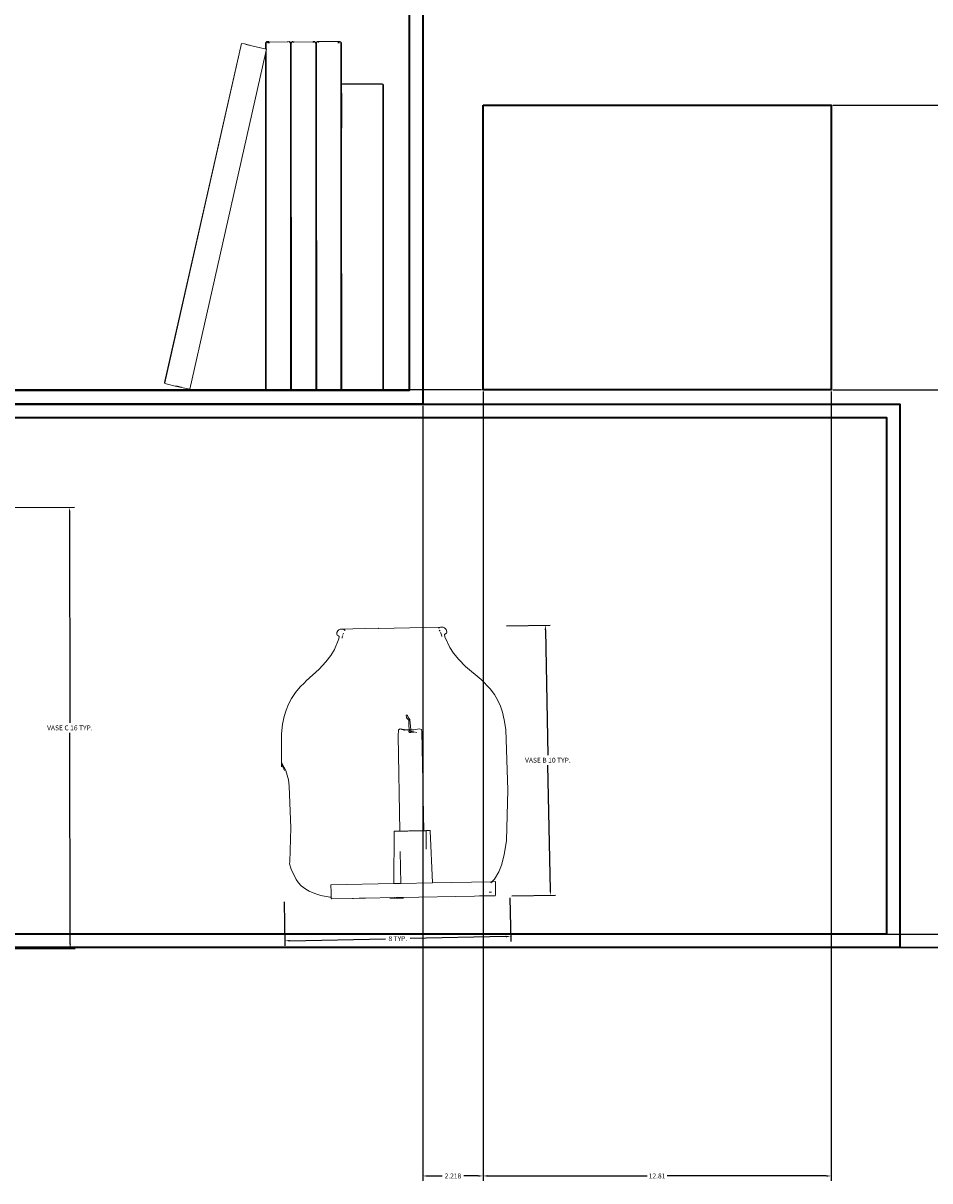
# Model space of a CAD drawing. Units: millimetres. Extents: x 446512 to 447461, y 70395 to 70610.
# Tile 6 of 39: x 446714 to 446748, y 70405 to 70447. Entities that reach past the tile are written whole.
import ezdxf

# ---------------------------------------------------------------- set-up
doc = ezdxf.new("R2010")
doc.units = ezdxf.units.MM
for name, color, linetype, lineweight in [('A-ANNO-DIMS', 2, 'Continuous', 18), ('A-FURN', 7, 'Continuous', 35), ('A-FURN-DECO', 8, 'Continuous', 13)]:
    doc.layers.add(name, color=color, linetype=linetype, lineweight=lineweight)
doc.styles.get("Standard").update_dxf_attribs({"font": 'arial.ttf'})
doc.dimstyles.get("Standard").update_dxf_attribs({"dimtxt": 0.18, "dimasz": 0.18, "dimexe": 0.18, "dimexo": 0.0625, "dimgap": 0.09, "dimtad": 0, "dimtih": 1, "dimtoh": 1, "dimdec": 4, "dimzin": 0, "dimdsep": 46, "dimtxsty": 'Standard', "dimcen": 0.09, "dimadec": 0, "dimazin": 0, "dimtfac": 1, "dimtdec": 4, "dimtofl": 0, "dimtmove": 0, "dimatfit": 3, "dimfxl": 1, "dimtolj": 1, "dimtzin": 0, "dimarcsym": 0})

# ---------------------------------------------------------------- blocks, each defined once
blk = doc.blocks.new('DECO-VASE-B')
for p, q in [((2.121, 9.752), (2.128, 9.807)), ((2.128, 9.807), (2.158, 9.87)), ((2.158, 9.87), (2.204, 9.914)), ((2.204, 9.914), (2.257, 9.937)), ((2.257, 9.937), (2.375, 9.928)), ((2.257, 9.937), (3.651, 9.937)), ((2.375, 9.928), (2.419, 9.892)), ((2.419, 9.892), (2.422, 9.871)), ((3.666, 9.936), (3.651, 9.937)), ((3.666, 9.936), (5.973, 9.937)), ((5.872, 9.93), (5.946, 9.933)), ((5.899, 9.917), (5.879, 9.893)), ((5.891, 9.829), (5.92, 9.807)), ((5.946, 9.933), (5.899, 9.917)), ((5.92, 9.807), (5.927, 9.787)), ((5.973, 9.937), (5.946, 9.933)), ((5.977, 9.937), (5.973, 9.937)), ((5.977, 9.937), (6.043, 9.936)), ((6.097, 9.911), (6.043, 9.936)), ((6.151, 9.85), (6.097, 9.911)), ((6.169, 9.807), (6.151, 9.85)), ((6.174, 9.743), (6.169, 9.807)), ((2.026, 9.184), (2.196, 9.575)), ((2.121, 9.752), (2.136, 9.719)), ((2.184, 9.693), (2.136, 9.719)), ((2.208, 9.658), (2.184, 9.693)), ((2.196, 9.575), (2.208, 9.658)), ((2.323, 9.65), (2.313, 9.594)), ((2.34, 9.701), (2.323, 9.65)), ((2.369, 9.787), (2.35, 9.732)), ((5.944, 9.737), (5.948, 9.727)), ((5.954, 9.711), (5.974, 9.652)), ((5.974, 9.652), (5.984, 9.593)), ((6.088, 9.658), (6.097, 9.677)), ((6.101, 9.575), (6.088, 9.658)), ((6.097, 9.677), (6.158, 9.717)), ((6.27, 9.184), (6.101, 9.575)), ((6.158, 9.717), (6.174, 9.743)), ((1.704, 8.737), (1.892, 8.976)), ((1.892, 8.976), (2.026, 9.184)), ((6.405, 8.976), (6.27, 9.184)), ((6.592, 8.737), (6.405, 8.976)), ((1.454, 8.473), (1.704, 8.737)), ((6.842, 8.473), (6.592, 8.737)), ((0.966, 8.05), (1.454, 8.473)), ((7.4, 7.989), (6.842, 8.473)), ((0.562, 7.63), (0.741, 7.837)), ((0.741, 7.837), (0.896, 7.989)), ((0.896, 7.989), (0.966, 8.05)), ((7.734, 7.63), (7.4, 7.989)), ((0.415, 7.419), (0.296, 7.204)), ((0.562, 7.63), (0.415, 7.419)), ((7.882, 7.419), (7.734, 7.63)), ((8.001, 7.204), (7.882, 7.419)), ((0.13, 6.762), (0.202, 6.985)), ((0.202, 6.985), (0.296, 7.204)), ((8.095, 6.985), (8.001, 7.204)), ((8.167, 6.762), (8.095, 6.985)), ((0.022, 6.129), (0.066, 6.478)), ((0.066, 6.478), (0.13, 6.762)), ((4.665, 6.727), (4.616, 6.724)), ((4.628, 6.627), (4.616, 6.724)), ((4.711, 6.536), (4.628, 6.627)), ((4.676, 6.66), (4.665, 6.727)), ((4.753, 6.557), (4.676, 6.66)), ((4.714, 6.371), (4.711, 6.536)), ((4.753, 6.557), (4.779, 6.182)), ((8.23, 6.478), (8.167, 6.762)), ((8.274, 6.129), (8.23, 6.478)), ((0.003, 5.065), (0.022, 6.129)), ((4.307, 5.974), (4.332, 6.194)), ((4.307, 2.461), (4.307, 5.974)), ((4.392, 6.222), (4.332, 6.194)), ((4.611, 6.182), (4.392, 6.222)), ((4.567, 6.159), (4.412, 6.207)), ((4.412, 6.207), (4.611, 6.182)), ((4.611, 6.182), (4.719, 6.182)), ((4.72, 6.153), (4.611, 6.182)), ((4.721, 6.111), (4.691, 6.12)), ((4.719, 6.182), (4.714, 6.371)), ((4.72, 6.153), (4.719, 6.182)), ((4.719, 6.182), (4.779, 6.182)), ((4.782, 6.137), (4.72, 6.153)), ((4.72, 6.143), (4.72, 6.149)), ((4.721, 6.111), (4.721, 6.13)), ((4.752, 6.101), (4.721, 6.111)), ((4.722, 6.089), (4.721, 6.111)), ((4.761, 6.087), (4.722, 6.089)), ((4.752, 6.101), (4.784, 6.098)), ((4.761, 6.087), (4.785, 6.086)), ((4.779, 6.182), (4.782, 6.137)), ((4.779, 6.182), (4.892, 6.182)), ((5.006, 6.08), (4.782, 6.137)), ((4.782, 6.129), (4.783, 6.109)), ((4.784, 6.098), (4.785, 6.086)), ((4.784, 6.098), (4.899, 6.089)), ((4.892, 6.182), (5.091, 6.212)), ((5.091, 6.212), (5.171, 6.181)), ((5.19, 6.109), (5.171, 6.181)), ((5.19, 6.109), (5.194, 2.461)), ((8.315, 3.894), (8.274, 6.129)), ((0, 4.992), (0.003, 5.065)), ((0.002, 4.989), (0, 4.992)), ((0, 4.911), (0.002, 4.989)), ((0.057, 4.898), (0.002, 4.989)), ((0.003, 5.065), (0.148, 4.769)), ((0.105, 4.769), (0.057, 4.898)), ((0.148, 4.769), (0.24, 4.424)), ((0.24, 4.424), (0.27, 4.187)), ((0.27, 4.187), (0.298, 2.664)), ((8.221, 2.044), (8.315, 3.894)), ((0.298, 2.664), (0.234, 1.404)), ((4.054, 0.538), (4.098, 2.454)), ((4.098, 2.454), (4.106, 2.461)), ((4.106, 2.461), (4.163, 2.461)), ((4.163, 2.461), (4.167, 2.461)), ((4.167, 2.461), (4.192, 2.461)), ((4.192, 2.461), (4.198, 2.461)), ((4.198, 2.461), (4.201, 2.461)), ((4.201, 2.461), (4.218, 2.461)), ((4.218, 2.461), (4.227, 2.461)), ((4.227, 2.461), (4.232, 2.461)), ((4.232, 2.461), (4.235, 2.461)), ((4.235, 2.461), (4.239, 2.461)), ((4.239, 2.461), (4.246, 2.461)), ((4.25, 2.461), (4.246, 2.461)), ((4.246, 2.461), (4.246, 2.454)), ((4.25, 2.461), (4.253, 2.461)), ((4.253, 2.461), (4.261, 2.461)), ((4.274, 2.461), (4.261, 2.461)), ((4.278, 2.461), (4.274, 2.461)), ((4.278, 2.461), (4.29, 2.461)), ((4.29, 2.461), (4.293, 2.461)), ((4.293, 2.461), (4.295, 2.461)), ((4.295, 2.461), (4.307, 2.461)), ((4.307, 2.454), (4.307, 2.461)), ((4.323, 2.461), (4.307, 2.461)), ((4.323, 2.461), (4.344, 2.461)), ((4.416, 2.461), (4.344, 2.461)), ((4.427, 2.461), (4.416, 2.461)), ((4.427, 2.461), (4.484, 2.461)), ((4.484, 2.461), (4.498, 2.461)), ((4.498, 2.461), (4.589, 2.461)), ((4.605, 2.461), (4.589, 2.461)), ((4.605, 2.461), (4.638, 2.461)), ((4.732, 2.461), (4.638, 2.461)), ((4.732, 2.461), (4.738, 2.461)), ((4.738, 2.461), (4.839, 2.461)), ((4.861, 2.461), (4.839, 2.461)), ((4.861, 2.461), (4.924, 2.461)), ((4.924, 2.461), (4.937, 2.461)), ((4.973, 2.461), (4.937, 2.461)), ((4.978, 2.461), (4.973, 2.461)), ((4.983, 2.461), (4.978, 2.461)), ((4.983, 2.461), (4.987, 2.461)), ((4.987, 2.461), (4.99, 2.461)), ((4.99, 2.461), (5.024, 2.461)), ((5.037, 2.461), (5.024, 2.461)), ((5.064, 2.461), (5.037, 2.461)), ((5.064, 2.461), (5.07, 2.461)), ((5.07, 2.461), (5.144, 2.461)), ((5.154, 2.461), (5.144, 2.461)), ((5.154, 2.461), (5.181, 2.461)), ((5.188, 2.461), (5.181, 2.461)), ((5.194, 2.461), (5.188, 2.461)), ((5.194, 2.461), (5.194, 2.454)), ((5.196, 2.461), (5.194, 2.461)), ((5.202, 2.461), (5.196, 2.461)), ((5.204, 2.461), (5.202, 2.461)), ((5.204, 2.461), (5.219, 2.461)), ((5.224, 2.461), (5.219, 2.461)), ((5.244, 2.461), (5.224, 2.461)), ((5.249, 2.461), (5.244, 2.461)), ((5.249, 2.461), (5.262, 2.461)), ((5.276, 2.461), (5.262, 2.461)), ((5.276, 2.461), (5.266, 1.782)), ((5.28, 2.461), (5.276, 2.461)), ((5.285, 2.461), (5.28, 2.461)), ((5.285, 2.461), (5.312, 2.461)), ((5.312, 2.461), (5.318, 2.461)), ((5.318, 2.461), (5.325, 2.461)), ((5.325, 2.461), (5.348, 2.461)), ((5.348, 2.461), (5.351, 2.461)), ((5.351, 2.461), (5.355, 2.461)), ((5.355, 2.461), (5.365, 2.461)), ((5.365, 2.461), (5.415, 2.461)), ((5.423, 2.454), (5.415, 2.461)), ((5.467, 0.538), (5.423, 2.454)), ((4.307, 0.538), (4.307, 1.712)), ((8.128, 1.516), (8.221, 2.044)), ((0.234, 1.404), (0.221, 1.331)), ((0.275, 1.141), (0.221, 1.331)), ((8.022, 1.141), (8.128, 1.516)), ((0.453, 0.752), (0.275, 1.141)), ((7.756, 0.627), (7.921, 0.896)), ((7.921, 0.896), (8.022, 1.141)), ((0.54, 0.627), (0.453, 0.752)), ((0.637, 0.522), (0.54, 0.627)), ((0.804, 0.392), (0.637, 0.522)), ((1.734, 0.266), (1.734, 0.538)), ((4.054, 0.538), (1.734, 0.538)), ((4.307, 0.538), (4.054, 0.538)), ((4.307, 0.538), (5.467, 0.538)), ((7.621, 0.538), (5.467, 0.538)), ((7.621, 0.499), (7.662, 0.538)), ((7.621, 0.538), (7.662, 0.538)), ((7.662, 0.538), (7.756, 0.627)), ((7.675, 0.538), (7.662, 0.538)), ((7.692, 0.538), (7.675, 0.538)), ((7.692, 0.538), (7.787, 0.538)), ((7.788, 0.049), (7.787, 0.538)), ((0.929, 0.318), (0.804, 0.392)), ((1.134, 0.226), (0.929, 0.318)), ((1.358, 0.154), (1.134, 0.226)), ((1.679, 0.085), (1.358, 0.154)), ((1.734, 0.078), (1.679, 0.085)), ((1.734, 0.078), (1.734, 0.266)), ((1.734, 0.049), (1.734, 0.078)), ((1.757, 0.021), (1.734, 0.049)), ((2.515, 0.021), (1.757, 0.021)), ((2.539, 0.023), (2.515, 0.021)), ((2.551, 0.021), (2.539, 0.023)), ((2.551, 0.021), (2.948, 0.021)), ((2.948, 0.021), (2.761, 0.023)), ((2.969, 0.024), (2.948, 0.021)), ((2.991, 0.021), (2.969, 0.024)), ((2.991, 0.021), (4.067, 0.021)), ((3.896, 0), (4.077, 0.018)), ((4.077, 0.018), (4.067, 0.021)), ((4.077, 0.018), (4.126, 0.021)), ((4.176, 0.018), (4.126, 0.021)), ((4.196, 0.021), (4.176, 0.018)), ((4.196, 0.021), (4.248, 0.018)), ((4.248, 0.018), (4.27, 0.021)), ((4.392, 0), (4.248, 0.018)), ((4.27, 0.021), (7.006, 0.021)), ((7.006, 0.021), (7.192, 0.022)), ((7.325, 0.021), (7.192, 0.022)), ((7.325, 0.021), (7.349, 0.022)), ((7.349, 0.022), (7.351, 0.022)), ((7.349, 0.022), (7.353, 0.022)), ((7.353, 0.022), (7.467, 0.021)), ((7.467, 0.021), (7.488, 0.022)), ((7.488, 0.022), (7.49, 0.022)), ((7.49, 0.022), (7.582, 0.021)), ((7.582, 0.021), (7.645, 0.021)), ((7.645, 0.021), (7.67, 0.021)), ((7.683, 0.021), (7.67, 0.021)), ((7.765, 0.021), (7.683, 0.021)), ((7.765, 0.021), (7.788, 0.049)), ((3.896, 0), (4.392, 0))]:
    blk.add_line(p, q)
blk = doc.blocks.new('*D9')
at = {"layer": 'A-ANNO-DIMS', "color": 0, "lineweight": -2, "transparency": 16777216}
for p, q in [((446732.091, 70425.219), (446733.698, 70425.249)), ((446733.522, 70425.066), (446733.609, 70420.461)), ((446733.703, 70415.491), (446733.616, 70420.095)), ((446732.279, 70415.284), (446733.887, 70415.314))]:
    blk.add_line(p, q, dxfattribs=at)
at = {"layer": 'A-ANNO-DIMS', "color": 0, "transparency": 16777216}
for points in [[(446733.552, 70425.067), (446733.492, 70425.065), (446733.518, 70425.246)], [(446733.733, 70415.491), (446733.673, 70415.49), (446733.707, 70415.311)]]:
    blk.add_solid(points, dxfattribs=at)
at = {"layer": 'Defpoints', "color": 0, "transparency": 16777216}
for p in [(446732.028, 70425.218), (446733.518, 70425.246), (446732.216, 70415.282)]:
    blk.add_point(p, dxfattribs=at)
at = {"layer": 'A-ANNO-DIMS', "color": 0, "transparency": 16777216, "insert": (446733.612, 70420.278), "char_height": 0.18, "attachment_point": 5}
blk.add_mtext('\\A1;VASE B 10 TYP.', dxfattribs=at)
blk = doc.blocks.new('*D10')
at = {"layer": 'A-ANNO-DIMS', "color": 0, "lineweight": -2, "transparency": 16777216}
for p, q in [((446723.904, 70415.063), (446723.934, 70413.455)), ((446732.217, 70415.22), (446732.248, 70413.612)), ((446724.111, 70413.638), (446727.629, 70413.705)), ((446732.064, 70413.789), (446728.546, 70413.722))]:
    blk.add_line(p, q, dxfattribs=at)
at = {"layer": 'A-ANNO-DIMS', "color": 0, "transparency": 16777216}
for points in [[(446724.11, 70413.668), (446724.111, 70413.608), (446723.931, 70413.635)], [(446732.064, 70413.819), (446732.065, 70413.759), (446732.244, 70413.792)]]:
    blk.add_solid(points, dxfattribs=at)
at = {"layer": 'Defpoints', "color": 0, "transparency": 16777216}
for p in [(446732.216, 70415.282), (446723.903, 70415.125), (446732.244, 70413.792)]:
    blk.add_point(p, dxfattribs=at)
at = {"layer": 'A-ANNO-DIMS', "color": 0, "transparency": 16777216, "insert": (446728.088, 70413.713), "char_height": 0.18, "attachment_point": 5}
blk.add_mtext('\\A1;8 TYP.', dxfattribs=at)
blk = doc.blocks.new('*D11')
at = {"layer": 'A-ANNO-DIMS', "color": 0, "lineweight": -2, "transparency": 16777216}
for p, q in [((446713.633, 70429.58), (446716.185, 70429.583)), ((446716.005, 70429.403), (446716.016, 70421.65)), ((446716.027, 70413.531), (446716.017, 70421.284)), ((446713.655, 70413.347), (446716.208, 70413.351))]:
    blk.add_line(p, q, dxfattribs=at)
at = {"layer": 'A-ANNO-DIMS', "color": 0, "transparency": 16777216}
for points in [[(446716.035, 70429.403), (446715.975, 70429.403), (446716.005, 70429.583)], [(446716.057, 70413.531), (446715.997, 70413.531), (446716.028, 70413.351)]]:
    blk.add_solid(points, dxfattribs=at)
at = {"layer": 'Defpoints', "color": 0, "transparency": 16777216}
for p in [(446713.57, 70429.58), (446716.005, 70429.583), (446713.593, 70413.347)]:
    blk.add_point(p, dxfattribs=at)
at = {"layer": 'A-ANNO-DIMS', "color": 0, "transparency": 16777216, "insert": (446716.016, 70421.467), "char_height": 0.18, "attachment_point": 5}
blk.add_mtext('\\A1;VASE C 16 TYP.', dxfattribs=at)
blk = doc.blocks.new('*D18')
at = {"layer": 'A-ANNO-DIMS', "color": 0, "lineweight": -2, "transparency": 16777216}
for p, q in [((446686.51, 70433.382), (446678.043, 70433.382)), ((446678.223, 70433.202), (446678.223, 70423.563)), ((446678.223, 70413.562), (446678.223, 70423.2)), ((446749.161, 70413.382), (446678.043, 70413.382))]:
    blk.add_line(p, q, dxfattribs=at)
at = {"layer": 'A-ANNO-DIMS', "color": 0, "transparency": 16777216}
for points in [[(446678.193, 70433.202), (446678.253, 70433.202), (446678.223, 70433.382)], [(446678.193, 70413.562), (446678.253, 70413.562), (446678.223, 70413.382)]]:
    blk.add_solid(points, dxfattribs=at)
at = {"layer": 'Defpoints', "color": 0, "transparency": 16777216}
for p in [(446678.223, 70433.382), (446686.573, 70433.382), (446749.223, 70413.382)]:
    blk.add_point(p, dxfattribs=at)
at = {"layer": 'A-ANNO-DIMS', "color": 0, "transparency": 16777216, "insert": (446678.223, 70423.382), "char_height": 0.18, "attachment_point": 5}
blk.add_mtext('\\A1;20', dxfattribs=at)
blk = doc.blocks.new('*D25')
at = {"layer": 'A-ANNO-DIMS', "color": 0, "lineweight": -2, "transparency": 16777216}
for p, q in [((446731.226, 70433.842), (446731.226, 70404.803)), ((446744.038, 70433.842), (446744.038, 70404.803)), ((446731.406, 70404.983), (446737.264, 70404.983)), ((446743.858, 70404.983), (446738, 70404.983))]:
    blk.add_line(p, q, dxfattribs=at)
at = {"layer": 'A-ANNO-DIMS', "color": 0, "transparency": 16777216}
for points in [[(446731.406, 70405.013), (446731.406, 70404.953), (446731.226, 70404.983)], [(446743.858, 70405.013), (446743.858, 70404.953), (446744.038, 70404.983)]]:
    blk.add_solid(points, dxfattribs=at)
at = {"layer": 'Defpoints', "color": 0, "transparency": 16777216}
for p in [(446731.226, 70433.905), (446744.038, 70433.905), (446744.038, 70404.983)]:
    blk.add_point(p, dxfattribs=at)
at = {"layer": 'A-ANNO-DIMS', "color": 0, "transparency": 16777216, "insert": (446737.632, 70404.983), "char_height": 0.18, "attachment_point": 5}
blk.add_mtext('\\A1;12.81', dxfattribs=at)
blk = doc.blocks.new('*D26')
at = {"layer": 'A-ANNO-DIMS', "color": 0, "lineweight": -2, "transparency": 16777216}
for p, q in [((446744.1, 70444.38), (446787.753, 70444.38)), ((446787.573, 70444.2), (446787.573, 70439.324)), ((446787.573, 70434.085), (446787.573, 70438.96)), ((446744.1, 70433.905), (446787.753, 70433.905))]:
    blk.add_line(p, q, dxfattribs=at)
at = {"layer": 'A-ANNO-DIMS', "color": 0, "transparency": 16777216}
for points in [[(446787.543, 70444.2), (446787.603, 70444.2), (446787.573, 70444.38)], [(446787.543, 70434.085), (446787.603, 70434.085), (446787.573, 70433.905)]]:
    blk.add_solid(points, dxfattribs=at)
at = {"layer": 'Defpoints', "color": 0, "transparency": 16777216}
for p in [(446744.038, 70444.38), (446787.573, 70444.38), (446744.038, 70433.905)]:
    blk.add_point(p, dxfattribs=at)
at = {"layer": 'A-ANNO-DIMS', "color": 0, "transparency": 16777216, "insert": (446787.573, 70439.142), "char_height": 0.18, "attachment_point": 5}
blk.add_mtext('\\A1;10.475', dxfattribs=at)
blk = doc.blocks.new('*D27')
at = {"layer": 'A-ANNO-DIMS', "color": 0, "lineweight": -2, "transparency": 16777216}
for p, q in [((446731.226, 70433.842), (446731.226, 70404.803)), ((446729.008, 70433.319), (446729.008, 70404.803)), ((446729.188, 70404.983), (446729.722, 70404.983)), ((446731.046, 70404.983), (446730.513, 70404.983))]:
    blk.add_line(p, q, dxfattribs=at)
at = {"layer": 'A-ANNO-DIMS', "color": 0, "transparency": 16777216}
for points in [[(446729.188, 70405.013), (446729.188, 70404.953), (446729.008, 70404.983)], [(446731.046, 70405.013), (446731.046, 70404.953), (446731.226, 70404.983)]]:
    blk.add_solid(points, dxfattribs=at)
at = {"layer": 'Defpoints', "color": 0, "transparency": 16777216}
for p in [(446731.226, 70433.905), (446729.008, 70433.382), (446731.226, 70404.983)]:
    blk.add_point(p, dxfattribs=at)
at = {"layer": 'A-ANNO-DIMS', "color": 0, "transparency": 16777216, "insert": (446730.117, 70404.983), "char_height": 0.18, "attachment_point": 5}
blk.add_mtext('\\A1;2.218', dxfattribs=at)
blk = doc.blocks.new('*D28')
at = {"layer": 'A-ANNO-DIMS', "color": 0, "lineweight": -2, "transparency": 16777216}
for p, q in [((446678.223, 70434.085), (446678.223, 70434.265)), ((446731.164, 70433.905), (446678.043, 70433.905)), ((446728.946, 70433.382), (446678.043, 70433.382)), ((446678.223, 70433.202), (446678.223, 70433.022))]:
    blk.add_line(p, q, dxfattribs=at)
at = {"layer": 'A-ANNO-DIMS', "color": 0, "transparency": 16777216}
for points in [[(446678.193, 70434.085), (446678.253, 70434.085), (446678.223, 70433.905)], [(446678.193, 70433.202), (446678.253, 70433.202), (446678.223, 70433.382)]]:
    blk.add_solid(points, dxfattribs=at)
at = {"layer": 'Defpoints', "color": 0, "transparency": 16777216}
for p in [(446731.226, 70433.905), (446678.223, 70433.382), (446729.008, 70433.382)]:
    blk.add_point(p, dxfattribs=at)
at = {"layer": 'A-ANNO-DIMS', "color": 0, "transparency": 16777216, "insert": (446678.223, 70433.643), "char_height": 0.18, "attachment_point": 5}
blk.add_mtext('\\A1;0.523', dxfattribs=at)
blk = doc.blocks.new('*D45')
at = {"layer": 'A-ANNO-DIMS', "color": 0, "lineweight": -2, "transparency": 16777216}
for p, q in [((446787.57348, 70414.06155), (446787.57348, 70414.24155)), ((446699.991325, 70413.88155), (446787.75348, 70413.88155)), ((446699.491325, 70413.38155), (446787.75348, 70413.38155)), ((446787.57348, 70413.20155), (446787.57348, 70413.02155))]:
    blk.add_line(p, q, dxfattribs=at)
at = {"layer": 'A-ANNO-DIMS', "color": 0, "transparency": 16777216}
for points in [[(446787.54348, 70414.06155), (446787.60348, 70414.06155), (446787.57348, 70413.88155)], [(446787.54348, 70413.20155), (446787.60348, 70413.20155), (446787.57348, 70413.38155)]]:
    blk.add_solid(points, dxfattribs=at)
at = {"layer": 'Defpoints', "color": 0, "transparency": 16777216}
for p in [(446699.928825, 70413.88155), (446699.428825, 70413.38155), (446787.57348, 70413.38155)]:
    blk.add_point(p, dxfattribs=at)
at = {"layer": 'A-ANNO-DIMS', "color": 0, "transparency": 16777216, "insert": (446787.57348, 70413.63155), "char_height": 0.18, "attachment_point": 5}
blk.add_mtext('\\A1;0.5', dxfattribs=at)

msp = doc.modelspace()

# ---------------------------------------------------------------- linework, layer by layer
at = {"layer": 'A-FURN'}
for p, q in [((446729.0084, 70453.3815), (446729.0084, 70433.3815)), ((446686.5728, 70433.3815), (446746.5728, 70433.3815)), ((446746.5728, 70433.3815), (446746.5728, 70413.3815)), ((446746.5728, 70413.3815), (446686.5728, 70413.3815))]:
    msp.add_line(p, q, dxfattribs=at)
for points in [[(446686.5728, 70453.3815), (446729.0084, 70453.3815), (446729.0084, 70433.3815), (446686.5728, 70433.3815)], [(446687.0728, 70452.8815), (446728.5084, 70452.8815), (446728.5084, 70433.8815), (446687.0728, 70433.8815)], [(446731.2264, 70444.3797), (446744.0375, 70444.3797), (446744.0375, 70433.9045), (446731.2264, 70433.9045)], [(446699.4288, 70433.3815), (446746.5728, 70433.3815), (446746.5728, 70413.3815), (446699.4288, 70413.3815)], [(446699.9288, 70432.8815), (446746.0728, 70432.8815), (446746.0728, 70413.8815), (446699.9288, 70413.8815)]]:
    msp.add_lwpolyline(points, close=True, dxfattribs=at)
at = {"layer": 'A-FURN-DECO'}
for p, q in [((446719.5038, 70434.1674), (446722.3274, 70446.649)), ((446722.3289, 70446.6487), (446719.5123, 70434.1574)), ((446722.3274, 70446.649), (446722.3289, 70446.6487)), ((446722.3289, 70446.6487), (446722.4379, 70446.6339)), ((446722.7137, 70446.5619), (446722.4379, 70446.6339)), ((446722.7137, 70446.5619), (446722.4904, 70446.6123)), ((446723.1964, 70446.4532), (446722.7137, 70446.5619)), ((446723.2156, 70446.4586), (446723.1964, 70446.4532)), ((446723.1964, 70446.4532), (446723.2457, 70446.4421)), ((446723.2156, 70446.4586), (446723.2218, 70446.4557)), ((446723.2206, 70446.2812), (446723.2459, 70446.3931)), ((446723.2364, 70446.6976), (446723.2218, 70446.6546)), ((446723.2218, 70446.6546), (446723.2218, 70446.4557)), ((446723.2459, 70446.4445), (446723.2218, 70446.4557)), ((446723.2218, 70446.4557), (446723.2218, 70446.4511)), ((446723.2364, 70446.6626), (446723.2364, 70446.6976)), ((446723.2364, 70446.6976), (446723.2459, 70446.6976)), ((446723.2459, 70446.3931), (446723.2451, 70433.8815)), ((446723.2459, 70446.4445), (446723.2457, 70446.4421)), ((446723.2548, 70446.44), (446723.2457, 70446.4421)), ((446723.2459, 70446.6976), (446723.2495, 70446.6996)), ((446723.2459, 70446.6976), (446723.2459, 70446.4445)), ((446723.2548, 70446.44), (446723.2459, 70446.4445)), ((446723.2459, 70446.4002), (446723.2548, 70446.44)), ((446723.2459, 70446.4002), (446723.2459, 70446.3931)), ((446723.2495, 70446.6996), (446723.2707, 70446.7119)), ((446723.2495, 70446.6996), (446723.2841, 70446.7051)), ((446723.2622, 70446.6976), (446723.2495, 70446.6996)), ((446723.2878, 70446.7032), (446723.2622, 70446.6976)), ((446723.2989, 70446.6976), (446723.2622, 70446.6976)), ((446723.3269, 70446.7119), (446723.2707, 70446.7119)), ((446723.2841, 70446.7051), (446723.2707, 70446.7119)), ((446723.2841, 70446.7051), (446723.2856, 70446.7053)), ((446723.2856, 70446.7053), (446723.3269, 70446.7119)), ((446723.2878, 70446.7032), (446723.2856, 70446.7053)), ((446723.2895, 70446.7036), (446723.2878, 70446.7032)), ((446723.3269, 70446.7119), (446723.2895, 70446.7036)), ((446723.2977, 70446.6982), (446723.2895, 70446.7036)), ((446723.2989, 70446.6976), (446723.2977, 70446.6982)), ((446723.3017, 70446.6982), (446723.2989, 70446.6976)), ((446723.3005, 70446.6553), (446723.2989, 70446.6976)), ((446723.3005, 70446.6976), (446723.2989, 70446.6976)), ((446723.3017, 70446.6982), (446723.3005, 70446.6976)), ((446723.3005, 70446.6553), (446723.3005, 70446.6976)), ((446723.3017, 70446.6982), (446723.3269, 70446.7119)), ((446723.3242, 70446.6986), (446723.3017, 70446.6982)), ((446723.3242, 70446.6986), (446723.324, 70446.6566)), ((446723.3269, 70446.7119), (446723.3242, 70446.6986)), ((446723.3274, 70446.6987), (446723.3242, 70446.6986)), ((446723.3242, 70446.6986), (446723.326, 70446.6567)), ((446723.3496, 70446.6991), (446723.3269, 70446.7119)), ((446723.3269, 70446.7119), (446723.3274, 70446.6987)), ((446723.3496, 70446.6991), (446723.3274, 70446.6987)), ((446723.3274, 70446.6987), (446723.329, 70446.6569)), ((446723.3522, 70446.6976), (446723.3496, 70446.6991)), ((446724.0441, 70446.7109), (446723.3522, 70446.6976)), ((446723.3522, 70446.6976), (446723.3534, 70446.6582)), ((446724.0236, 70446.6944), (446724.0235, 70446.6976)), ((446724.0456, 70446.7119), (446724.0441, 70446.7109)), ((446724.0473, 70446.711), (446724.0441, 70446.7109)), ((446724.045, 70446.6956), (446724.0451, 70446.6976)), ((446724.0456, 70446.7119), (446724.0473, 70446.711)), ((446724.0473, 70446.711), (446724.1018, 70446.7119)), ((446724.0484, 70446.6958), (446724.0485, 70446.6976)), ((446724.0818, 70446.6976), (446724.1104, 70446.6976)), ((446724.108, 70446.7015), (446724.0912, 70446.7043)), ((446724.108, 70446.7015), (446724.1018, 70446.7119)), ((446724.1318, 70446.6976), (446724.108, 70446.7015)), ((446724.1104, 70446.6976), (446724.108, 70446.7015)), ((446724.1104, 70446.6976), (446724.1318, 70446.6976)), ((446724.136, 70446.6546), (446724.1104, 70446.6976)), ((446724.1361, 70446.6976), (446724.1318, 70446.6976)), ((446724.1318, 70446.6976), (446724.1507, 70446.6546)), ((446724.1331, 70433.8845), (446724.136, 70446.6546)), ((446724.1507, 70446.6546), (446724.1361, 70446.6976)), ((446724.1507, 70446.6546), (446724.1361, 70433.8912)), ((446724.1507, 70446.6546), (446724.1695, 70446.6976)), ((446724.1507, 70433.9245), (446724.1507, 70446.6546)), ((446724.1695, 70433.8815), (446724.1507, 70446.6546)), ((446724.1653, 70433.8815), (446724.1507, 70446.6546)), ((446724.1658, 70446.6546), (446724.1707, 70446.663)), ((446724.1739, 70433.8815), (446724.1658, 70446.6546)), ((446724.1977, 70446.7023), (446724.1695, 70446.6976)), ((446724.1707, 70446.663), (446724.1695, 70446.6625)), ((446724.1707, 70446.663), (446724.191, 70446.6976)), ((446724.1977, 70446.7023), (446724.191, 70446.6976)), ((446724.2115, 70446.7119), (446724.1977, 70446.7023)), ((446724.2175, 70446.7055), (446724.1977, 70446.7023)), ((446724.2115, 70446.7119), (446724.2175, 70446.7055)), ((446724.2543, 70446.7111), (446724.2115, 70446.7119)), ((446724.2273, 70446.7072), (446724.2175, 70446.7055)), ((446724.2175, 70446.7055), (446724.2251, 70446.6976)), ((446724.2251, 70446.6976), (446724.2293, 70446.6976)), ((446724.2293, 70446.6976), (446724.24, 70446.7034)), ((446724.2293, 70446.6976), (446724.2528, 70446.6976)), ((446724.2528, 70446.6976), (446724.2532, 70446.6994)), ((446724.2595, 70446.6976), (446724.2528, 70446.6976)), ((446724.2543, 70446.7111), (446724.2558, 70446.7119)), ((446724.2558, 70446.7119), (446724.2572, 70446.7111)), ((446724.9632, 70446.6984), (446724.2572, 70446.7111)), ((446724.9632, 70446.6984), (446724.9718, 70446.7119)), ((446724.9772, 70446.6982), (446724.9632, 70446.6984)), ((446724.9718, 70446.7119), (446725.0347, 70446.7119)), ((446724.9768, 70446.7004), (446724.9772, 70446.6982)), ((446725.0107, 70446.6976), (446724.9772, 70446.6982)), ((446725.0399, 70446.6976), (446725.0031, 70446.7056)), ((446725.0399, 70446.6976), (446725.0347, 70446.7119)), ((446725.0454, 70446.6916), (446725.0399, 70446.6976)), ((446725.0649, 70446.6546), (446725.0454, 70446.6916)), ((446725.0795, 70446.6546), (446725.0454, 70446.6916)), ((446725.0795, 70446.6546), (446725.0644, 70433.9245)), ((446725.0645, 70436.4682), (446725.0795, 70446.6546)), ((446725.0645, 70436.4682), (446725.0649, 70446.6546)), ((446725.0795, 70433.9245), (446725.0946, 70446.6546)), ((446725.0946, 70446.6546), (446725.0941, 70446.6976)), ((446725.0941, 70446.6976), (446725.0971, 70446.6976)), ((446725.0946, 70446.6546), (446725.0971, 70446.6976)), ((446725.0946, 70446.6546), (446725.0957, 70444.9228)), ((446725.1301, 70446.7119), (446725.0971, 70446.6976)), ((446725.0971, 70446.6976), (446725.0984, 70446.6976)), ((446725.1393, 70446.7047), (446725.0984, 70446.6976)), ((446725.1301, 70446.7119), (446725.9475, 70446.7119)), ((446725.1582, 70446.6976), (446725.1817, 70446.6976)), ((446725.1817, 70446.6976), (446725.1818, 70446.6958)), ((446725.1857, 70446.6956), (446725.1855, 70446.6982)), ((446725.2036, 70446.6976), (446725.2099, 70446.6976)), ((446725.2099, 70446.6942), (446725.2099, 70446.6976)), ((446725.8915, 70446.6976), (446725.8885, 70446.6576)), ((446725.9062, 70446.6976), (446725.9011, 70446.6569)), ((446725.9062, 70446.6976), (446725.9042, 70446.6567)), ((446725.9062, 70446.6566), (446725.9062, 70446.6976)), ((446725.9297, 70446.6553), (446725.9297, 70446.6976)), ((446725.9327, 70446.6552), (446725.9339, 70446.6976)), ((446725.9778, 70446.7001), (446725.9475, 70446.7119)), ((446725.9605, 70446.7028), (446725.9625, 70446.7014)), ((446725.9625, 70446.7014), (446725.9778, 70446.7001)), ((446725.9778, 70446.7001), (446725.968, 70446.6976)), ((446725.9843, 70446.6976), (446725.9778, 70446.7001)), ((446725.9843, 70446.6976), (446725.9852, 70433.8815)), ((446725.9895, 70446.6976), (446725.9843, 70446.6976)), ((446725.9938, 70446.6976), (446725.9895, 70446.6976)), ((446725.9895, 70446.6976), (446725.9938, 70446.6879)), ((446726.0084, 70446.6546), (446725.9938, 70446.6976)), ((446725.9938, 70446.6976), (446725.9938, 70446.6879)), ((446725.9938, 70446.6879), (446725.9938, 70446.6626)), ((446725.9938, 70446.6879), (446726.0084, 70446.6546)), ((446726.0084, 70433.9245), (446726.0084, 70446.6546)), ((446723.2206, 70446.2812), (446721.0609, 70436.7046)), ((446723.2206, 70446.2812), (446723.2218, 70433.9245)), ((446726.0084, 70433.9245), (446726.0202, 70445.1064)), ((446726.0198, 70445.1428), (446726.0231, 70445.1428)), ((446726.0202, 70445.1064), (446726.0198, 70445.1428)), ((446726.0202, 70445.1064), (446726.0231, 70445.1428)), ((446726.0202, 70445.1064), (446726.0224, 70444.5504)), ((446726.0561, 70445.155), (446726.0231, 70445.1428)), ((446726.0625, 70445.1428), (446726.0231, 70445.1428)), ((446726.0561, 70445.155), (446726.0668, 70445.1428)), ((446727.4719, 70445.155), (446726.0561, 70445.155)), ((446726.0885, 70445.1428), (446726.0561, 70445.155)), ((446726.0668, 70445.1428), (446726.0625, 70445.1428)), ((446726.0701, 70445.1428), (446726.0668, 70445.1428)), ((446726.0668, 70445.1428), (446726.0682, 70445.1428)), ((446726.0682, 70445.1428), (446726.0701, 70445.1428)), ((446726.0885, 70445.1428), (446726.0701, 70445.1428)), ((446726.0885, 70445.1428), (446726.1, 70445.1428)), ((446726.1, 70445.1428), (446726.1028, 70445.1428)), ((446726.1028, 70445.1428), (446727.4542, 70445.1428)), ((446727.4542, 70445.1428), (446727.4719, 70445.155)), ((446727.474, 70445.1524), (446727.4542, 70445.1428)), ((446727.4542, 70445.1428), (446727.4736, 70445.1428)), ((446727.4719, 70445.155), (446727.474, 70445.155)), ((446727.4736, 70445.1428), (446727.474, 70445.1524)), ((446727.4763, 70445.1428), (446727.4736, 70445.1428)), ((446727.474, 70445.1524), (446727.474, 70445.155)), ((446727.5087, 70445.155), (446727.474, 70445.155)), ((446727.504, 70445.1496), (446727.474, 70445.155)), ((446727.4763, 70445.1428), (446727.474, 70445.1524)), ((446727.4816, 70445.1428), (446727.474, 70445.1524)), ((446727.4763, 70445.1428), (446727.4816, 70445.1428)), ((446727.4981, 70445.1428), (446727.4816, 70445.1428)), ((446727.4981, 70445.1428), (446727.504, 70445.1496)), ((446727.4981, 70445.1428), (446727.5334, 70445.1448)), ((446727.504, 70445.1496), (446727.5087, 70445.155)), ((446727.5334, 70445.1448), (446727.504, 70445.1496)), ((446727.5334, 70445.1448), (446727.5087, 70445.155)), ((446727.5382, 70445.1428), (446727.5334, 70445.1448)), ((446727.5382, 70433.8815), (446727.5382, 70445.1428)), ((446727.5417, 70445.1428), (446727.5382, 70445.1428)), ((446727.545, 70445.1428), (446727.5417, 70445.1428)), ((446727.5417, 70445.1428), (446727.545, 70445.1346)), ((446727.5565, 70445.1064), (446727.545, 70445.1428)), ((446727.545, 70445.1428), (446727.545, 70445.1346)), ((446727.545, 70445.1346), (446727.545, 70445.1132)), ((446727.545, 70445.1346), (446727.5565, 70445.1064)), ((446727.5565, 70433.9158), (446727.5565, 70445.1064)), ((446725.0957, 70444.9228), (446725.0795, 70433.9245)), ((446725.0957, 70444.9228), (446725.1027, 70433.8815)), ((446726.0224, 70444.5504), (446726.0197, 70442.4956)), ((446726.0197, 70442.4956), (446726.0084, 70433.9245)), ((446726.0191, 70433.8892), (446726.0197, 70442.4956)), ((446726.0197, 70442.4956), (446726.0266, 70433.8815)), ((446720.4348, 70433.9283), (446721.0609, 70436.7046)), ((446721.0609, 70436.7046), (446720.4367, 70433.9278)), ((446725.0644, 70433.9245), (446725.0645, 70436.4682)), ((446719.5038, 70434.1674), (446719.5077, 70434.1372)), ((446719.5077, 70434.1372), (446719.5123, 70434.1574)), ((446719.5077, 70434.1372), (446719.5092, 70434.1369)), ((446719.5123, 70434.1574), (446719.5092, 70434.1369)), ((446719.6044, 70434.1154), (446719.5092, 70434.1369)), ((446719.6044, 70434.1154), (446719.8948, 70434.0402)), ((446719.8948, 70434.0402), (446719.9722, 70434.0325)), ((446720.4196, 70433.9219), (446719.8948, 70434.0402)), ((446720.116, 70434.0001), (446719.9722, 70434.0325)), ((446720.116, 70434.0001), (446720.119, 70433.9991)), ((446720.4196, 70433.9219), (446720.3844, 70433.9379)), ((446720.4196, 70433.9219), (446720.4208, 70433.9314)), ((446720.4196, 70433.9219), (446720.4348, 70433.9283)), ((446720.4367, 70433.9278), (446720.4348, 70433.9283)), ((446723.2218, 70433.9245), (446723.2364, 70433.8815)), ((446723.2364, 70433.8912), (446723.2218, 70433.9245)), ((446723.2364, 70433.8815), (446723.2364, 70433.8912)), ((446723.2407, 70433.8815), (446723.2364, 70433.8912)), ((446723.2364, 70433.8815), (446723.2407, 70433.8815)), ((446723.2451, 70433.8815), (446723.2407, 70433.8815)), ((446723.2451, 70433.8815), (446724.1331, 70433.8815)), ((446724.1361, 70433.8912), (446724.1331, 70433.8845)), ((446724.1331, 70433.8815), (446724.1331, 70433.8845)), ((446724.1331, 70433.8815), (446724.1361, 70433.8815)), ((446724.1361, 70433.8815), (446724.1507, 70433.9245)), ((446724.1507, 70433.9245), (446724.1361, 70433.8912)), ((446724.1361, 70433.8912), (446724.1361, 70433.8815)), ((446724.1653, 70433.8815), (446724.1361, 70433.8815)), ((446724.1695, 70433.8815), (446724.1653, 70433.8815)), ((446724.1695, 70433.8815), (446724.1739, 70433.8815)), ((446725.0563, 70433.8815), (446724.1739, 70433.8815)), ((446725.0607, 70433.905), (446725.0563, 70433.8815)), ((446725.0607, 70433.8815), (446725.0563, 70433.8815)), ((446725.0644, 70433.9245), (446725.0607, 70433.905)), ((446725.0607, 70433.8815), (446725.0607, 70433.905)), ((446725.0649, 70433.8815), (446725.0607, 70433.8815)), ((446725.0644, 70433.9245), (446725.0649, 70433.8815)), ((446725.0941, 70433.8815), (446725.0649, 70433.8815)), ((446725.0795, 70433.9245), (446725.0941, 70433.8815)), ((446725.0941, 70433.8912), (446725.0795, 70433.9245)), ((446725.0941, 70433.8815), (446725.0941, 70433.8912)), ((446725.0984, 70433.8815), (446725.0941, 70433.8912)), ((446725.0941, 70433.8815), (446725.0984, 70433.8815)), ((446725.1027, 70433.8815), (446725.0984, 70433.8815)), ((446725.1027, 70433.8815), (446725.9852, 70433.8815)), ((446725.9895, 70433.8815), (446725.9852, 70433.8815)), ((446725.9938, 70433.8912), (446725.9895, 70433.8815)), ((446725.9895, 70433.8815), (446725.9938, 70433.8815)), ((446725.9938, 70433.8815), (446726.0084, 70433.9245)), ((446726.0084, 70433.9245), (446725.9938, 70433.8912)), ((446725.9938, 70433.9166), (446725.9938, 70433.8912)), ((446725.9938, 70433.8912), (446725.9938, 70433.8815)), ((446726.0191, 70433.8815), (446725.9938, 70433.8815)), ((446726.0084, 70433.9158), (446726.0084, 70433.9245)), ((446726.0084, 70433.9158), (446726.0191, 70433.8815)), ((446726.0191, 70433.8892), (446726.0084, 70433.9158)), ((446726.0191, 70433.8815), (446726.0191, 70433.8892)), ((446726.0223, 70433.8815), (446726.0191, 70433.8892)), ((446726.0223, 70433.8815), (446726.0191, 70433.8815)), ((446726.0266, 70433.8815), (446726.0223, 70433.8815)), ((446727.5382, 70433.8815), (446726.0266, 70433.8815)), ((446727.5426, 70433.8815), (446727.5382, 70433.8815)), ((446727.545, 70433.8876), (446727.5426, 70433.8815)), ((446727.5457, 70433.8815), (446727.5426, 70433.8815)), ((446727.5565, 70433.9158), (446727.545, 70433.8876)), ((446727.545, 70433.8876), (446727.5457, 70433.8815)), ((446727.5457, 70433.8815), (446727.5565, 70433.9158)), ((446731.5111, 70415.4289), (446731.4543, 70415.4285)), ((446731.5383, 70415.4289), (446731.5111, 70415.4289))]:
    msp.add_line(p, q, dxfattribs=at)

# ---------------------------------------------------------------- block references
at = {"layer": 'A-FURN-DECO', "rotation": 1.084701018374711}
msp.add_blockref('DECO-VASE-B', (446723.9029, 70415.1253), dxfattribs=at)

# ---------------------------------------------------------------- dimensions: what is measured, and where the dimension line sits
at = {"layer": 'A-ANNO-DIMS'}
for base, p1, p2, override, picture, middle in [((446787.5735, 70444.3797), (446744.0375, 70433.9045), (446744.0375, 70444.3797), {"dimdec": 3, "dimlfac": 1, "dimrnd": 0, "dimzin": 0, "dimdsep": 46, "dimlunit": 2}, '*D26', (446787.5735, 70439.1421)), ((446678.2228, 70433.3815), (446731.2264, 70433.9045), (446729.0084, 70433.3815), {"dimdec": 3, "dimlfac": 1, "dimrnd": 0, "dimzin": 0, "dimdsep": 46, "dimlunit": 2}, '*D28', (446678.2228, 70433.643)), ((446678.2228, 70433.3815), (446749.2235, 70413.3815), (446686.5728, 70433.3815), {"dimdec": 0, "dimlfac": 1, "dimrnd": 0, "dimzin": 0, "dimdsep": 46, "dimlunit": 2}, '*D18', (446678.2228, 70423.3815)), ((446787.5735, 70413.3815), (446699.9288, 70413.8815), (446699.4288, 70413.3815), {"dimdec": 1, "dimlfac": 1, "dimrnd": 0, "dimzin": 0, "dimdsep": 46, "dimlunit": 2}, '*D45', (446787.5735, 70413.6315))]:
    dim = msp.add_linear_dim(base=base, p1=p1, p2=p2, angle=90, dimstyle='Standard', override=override, dxfattribs=at)
    dim.commit()
    dim.dimension.update_dxf_attribs({"geometry": picture, "text_midpoint": middle})
for base, p1, p2, override, picture, middle in [((446731.2264, 70404.9832), (446729.0084, 70433.3815), (446731.2264, 70433.9045), {"dimdec": 3, "dimlfac": 1, "dimrnd": 0, "dimzin": 0, "dimdsep": 46, "dimlunit": 2}, '*D27', (446730.1174, 70404.9832)), ((446744.0375, 70404.9832), (446731.2264, 70433.9045), (446744.0375, 70433.9045), {"dimdec": 2, "dimlfac": 1, "dimrnd": 0, "dimzin": 0, "dimdsep": 46, "dimlunit": 2}, '*D25', (446737.632, 70404.9832))]:
    dim = msp.add_linear_dim(base=base, p1=p1, p2=p2, dimstyle='Standard', override=override, dxfattribs=at)
    dim.commit()
    dim.dimension.update_dxf_attribs({"geometry": picture, "text_midpoint": middle})
for base, p1, p2, angle, text, picture, middle in [((446716.0052, 70429.5831), (446713.5926, 70413.3472), (446713.5703, 70429.5798), 90.07882, 'VASE C <> TYP.', '*D11', (446716.0164, 70421.4668)), ((446733.5184, 70425.246), (446732.2162, 70415.2825), (446732.0281, 70425.2178), 91.0847, 'VASE B <> TYP.', '*D9', (446733.6125, 70420.2783)), ((446732.2445, 70413.7922), (446723.9026, 70415.125), (446732.2162, 70415.2825), 1.0847, '<> TYP.', '*D10', (446728.0877, 70413.7135))]:
    dim = msp.add_linear_dim(base=base, p1=p1, p2=p2, angle=angle, text=text, dimstyle='Standard', override={"dimdec": 0, "dimlfac": 1, "dimrnd": 0, "dimzin": 0, "dimdsep": 46, "dimlunit": 2}, dxfattribs=at)
    dim.commit()
    dim.dimension.update_dxf_attribs({"geometry": picture, "text_midpoint": middle})

doc.saveas('drawing.dxf')
